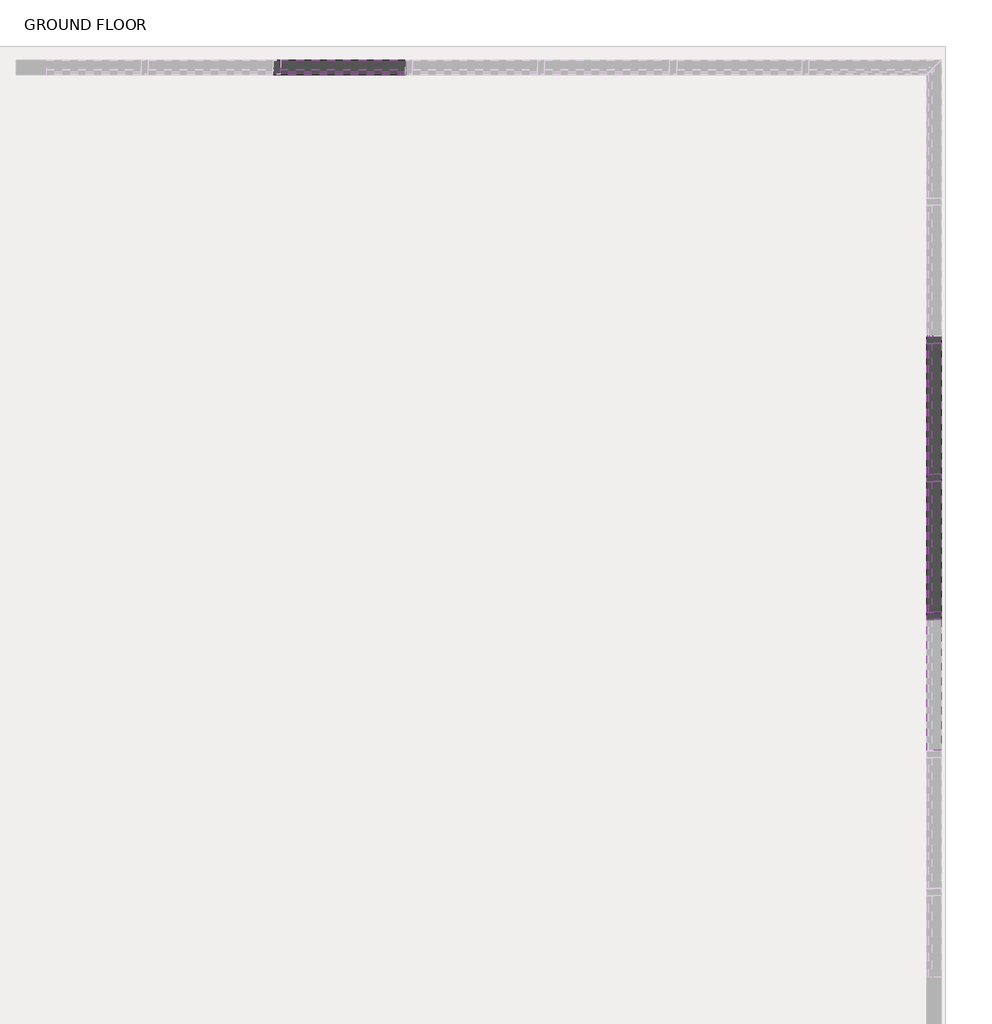
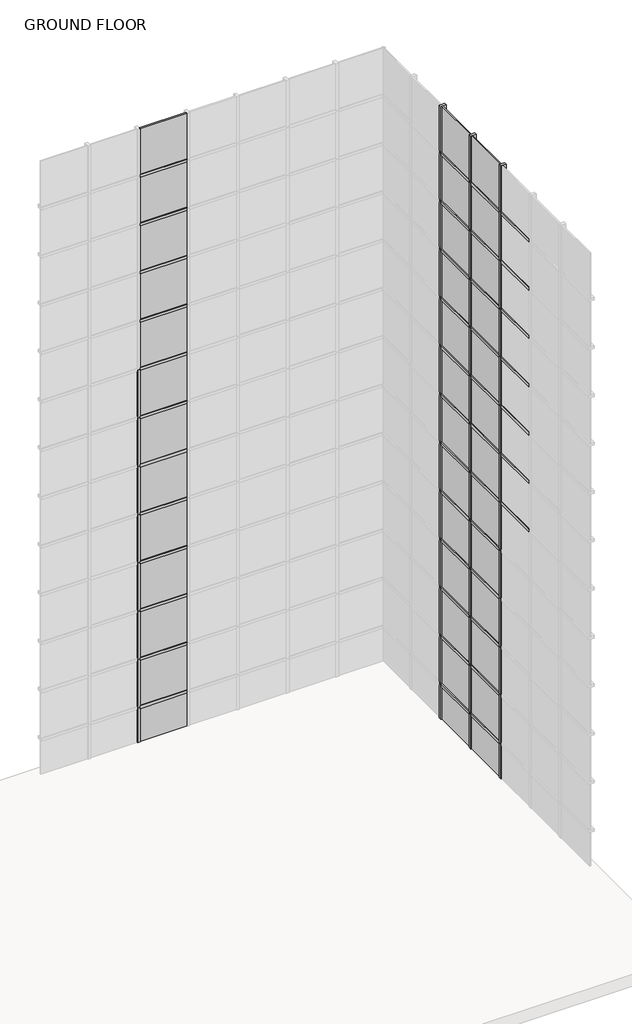
# One storey, part 12 of 16: 90 members, 39 plates.
"""IFC4 building model written with IfcOpenShell, lengths in millimetres."""

from ifc_helpers import new_model, si_unit, origin, place, context, project, spatial, transform, mapped, element, save
from components import member_d518c94e, member_b860638c, member_31fee25f, member_49b1bc66, system_panel_glazed_5cba32e5, system_panel_glazed_49652e9e

model = new_model("IFC4")

# Units and contexts
model_context = context("Model", 3, world=origin())
ifc_project = project(units=[si_unit("LENGTHUNIT", "METRE", prefix="MILLI")], contexts=[model_context])

# Site, building, storey
site = spatial("IfcSite", under=ifc_project)
building = spatial("IfcBuilding", under=site)
storey = spatial("IfcBuildingStorey", under=building, Name="GROUND FLOOR", Elevation=0.0)

# Members
placement = place(None, origin())
member_shape = member_d518c94e(model_context)
element("IfcMember", 1, ObjectType="Rectangular Mullion : 2.5\" x 5\" rectangular", at=placement, inside=storey, context=model_context, shape_type="MappedRepresentation", body=[
    mapped(member_shape, transform((198.8520927, 6370.2261968, 1168.8884615), x_axis=(0.0, 0.0, 1.0), y_axis=(0.0, 1.0, 0.0), z_axis=(-1.0, 0.0, 0.0))),
])
element("IfcMember", 2, ObjectType="Rectangular Mullion : 2.5\" x 5\" rectangular", at=placement, inside=storey, context=model_context, shape_type="MappedRepresentation", body=[
    mapped(member_shape, transform((198.8520927, 6370.2261968, 2369.5269231), x_axis=(0.0, 0.0, 1.0), y_axis=(0.0, 1.0, 0.0), z_axis=(-1.0, 0.0, 0.0))),
])
element("IfcMember", 3, ObjectType="Rectangular Mullion : 2.5\" x 5\" rectangular", at=placement, inside=storey, context=model_context, shape_type="MappedRepresentation", body=[
    mapped(member_shape, transform((198.8520927, 6370.2261968, 3570.1653846), x_axis=(0.0, 0.0, 1.0), y_axis=(0.0, 1.0, 0.0), z_axis=(-1.0, 0.0, 0.0))),
])
element("IfcMember", 4, ObjectType="Rectangular Mullion : 2.5\" x 5\" rectangular", at=placement, inside=storey, context=model_context, shape_type="MappedRepresentation", body=[
    mapped(member_shape, transform((198.8520927, 6370.2261968, 4770.8038462), x_axis=(0.0, 0.0, 1.0), y_axis=(0.0, 1.0, 0.0), z_axis=(-1.0, 0.0, 0.0))),
])
element("IfcMember", 5, ObjectType="Rectangular Mullion : 2.5\" x 5\" rectangular", at=placement, inside=storey, context=model_context, shape_type="MappedRepresentation", body=[
    mapped(member_shape, transform((198.8520927, 6370.2261968, 5971.4423077), x_axis=(0.0, 0.0, 1.0), y_axis=(0.0, 1.0, 0.0), z_axis=(-1.0, 0.0, 0.0))),
])
element("IfcMember", 6, ObjectType="Rectangular Mullion : 2.5\" x 5\" rectangular", at=placement, inside=storey, context=model_context, shape_type="MappedRepresentation", body=[
    mapped(member_shape, transform((198.8520927, 6370.2261968, 7172.0807692), x_axis=(0.0, 0.0, 1.0), y_axis=(0.0, 1.0, 0.0), z_axis=(-1.0, 0.0, 0.0))),
])
element("IfcMember", 7, ObjectType="Rectangular Mullion : 2.5\" x 5\" rectangular", at=placement, inside=storey, context=model_context, shape_type="MappedRepresentation", body=[
    mapped(member_shape, transform((198.8520927, 6370.2261968, 8372.7192308), x_axis=(0.0, 0.0, 1.0), y_axis=(0.0, 1.0, 0.0), z_axis=(-1.0, 0.0, 0.0))),
])
element("IfcMember", 8, ObjectType="Rectangular Mullion : 2.5\" x 5\" rectangular", at=placement, inside=storey, context=model_context, shape_type="MappedRepresentation", body=[
    mapped(member_shape, transform((198.8520927, 6370.2261968, 9573.3576923), x_axis=(0.0, 0.0, 1.0), y_axis=(0.0, 1.0, 0.0), z_axis=(-1.0, 0.0, 0.0))),
])
element("IfcMember", 9, ObjectType="Rectangular Mullion : 2.5\" x 5\" rectangular", at=placement, inside=storey, context=model_context, shape_type="MappedRepresentation", body=[
    mapped(member_shape, transform((198.8520927, 6370.2261968, 10773.9961538), x_axis=(0.0, 0.0, 1.0), y_axis=(0.0, 1.0, 0.0), z_axis=(-1.0, 0.0, 0.0))),
])
element("IfcMember", 10, ObjectType="Rectangular Mullion : 2.5\" x 5\" rectangular", at=placement, inside=storey, context=model_context, shape_type="MappedRepresentation", body=[
    mapped(member_shape, transform((198.8520927, 6370.2261968, 11974.6346154), x_axis=(0.0, 0.0, 1.0), y_axis=(0.0, 1.0, 0.0), z_axis=(-1.0, 0.0, 0.0))),
])
element("IfcMember", 11, ObjectType="Rectangular Mullion : 2.5\" x 5\" rectangular", at=placement, inside=storey, context=model_context, shape_type="MappedRepresentation", body=[
    mapped(member_shape, transform((198.8520927, 6370.2261968, 13175.2730769), x_axis=(0.0, 0.0, 1.0), y_axis=(0.0, 1.0, 0.0), z_axis=(-1.0, 0.0, 0.0))),
])
element("IfcMember", 12, ObjectType="Rectangular Mullion : 2.5\" x 5\" rectangular", at=placement, inside=storey, context=model_context, shape_type="MappedRepresentation", body=[
    mapped(member_shape, transform((198.8520927, 6370.2261968, 14375.9115385), x_axis=(0.0, 0.0, 1.0), y_axis=(0.0, 1.0, 0.0), z_axis=(-1.0, 0.0, 0.0))),
])
member_2_shape = member_b860638c(model_context)
element("IfcMember", 13, ObjectType="Rectangular Mullion : 2.5\" x 5\" rectangular", at=placement, inside=storey, context=model_context, shape_type="MappedRepresentation", body=[
    mapped(member_2_shape, transform((5962.6982466, 1532.7961967, 0.0), x_axis=(0.0, 1.0, 0.0), y_axis=(1.0, 0.0, 0.0), z_axis=(0.0, 0.0, -1.0))),
])
element("IfcMember", 14, ObjectType="Rectangular Mullion : 2.5\" x 5\" rectangular", at=placement, inside=storey, context=model_context, shape_type="MappedRepresentation", body=[
    mapped(member_2_shape, transform((5962.6982466, 2750.0911967, 0.0), x_axis=(0.0, 1.0, 0.0), y_axis=(1.0, 0.0, 0.0), z_axis=(0.0, 0.0, -1.0))),
])
element("IfcMember", 15, ObjectType="Rectangular Mullion : 2.5\" x 5\" rectangular", at=placement, inside=storey, context=model_context, shape_type="MappedRepresentation", body=[
    mapped(member_2_shape, transform((5962.6982466, 3967.3861966, 0.0), x_axis=(0.0, 1.0, 0.0), y_axis=(1.0, 0.0, 0.0), z_axis=(0.0, 0.0, -1.0))),
])
element("IfcMember", 16, ObjectType="Rectangular Mullion : 2.5\" x 5\" rectangular", at=placement, inside=storey, context=model_context, shape_type="MappedRepresentation", body=[
    mapped(member_2_shape, transform((167.1020927, 6370.2261968, 0.0), x_axis=(-1.0, 0.0, 0.0), y_axis=(0.0, 1.0, 0.0), z_axis=(0.0, 0.0, -1.0))),
])
member_3_shape = member_31fee25f(model_context)
element("IfcMember", 17, ObjectType="Rectangular Mullion : 2.5\" x 5\" rectangular", at=placement, inside=storey, context=model_context, shape_type="MappedRepresentation", body=[
    mapped(member_3_shape, transform((5962.6982466, 1532.7961967, 1168.8884615), x_axis=(0.0, 1.0, 0.0), y_axis=(1.0, 0.0, 0.0), z_axis=(0.0, 0.0, -1.0))),
])
element("IfcMember", 18, ObjectType="Rectangular Mullion : 2.5\" x 5\" rectangular", at=placement, inside=storey, context=model_context, shape_type="MappedRepresentation", body=[
    mapped(member_3_shape, transform((5962.6982466, 2750.0911967, 1168.8884615), x_axis=(0.0, 1.0, 0.0), y_axis=(1.0, 0.0, 0.0), z_axis=(0.0, 0.0, -1.0))),
])
element("IfcMember", 19, ObjectType="Rectangular Mullion : 2.5\" x 5\" rectangular", at=placement, inside=storey, context=model_context, shape_type="MappedRepresentation", body=[
    mapped(member_3_shape, transform((5962.6982466, 3967.3861966, 1168.8884615), x_axis=(0.0, 1.0, 0.0), y_axis=(1.0, 0.0, 0.0), z_axis=(0.0, 0.0, -1.0))),
])
element("IfcMember", 20, ObjectType="Rectangular Mullion : 2.5\" x 5\" rectangular", at=placement, inside=storey, context=model_context, shape_type="MappedRepresentation", body=[
    mapped(member_3_shape, transform((5962.6982466, 1532.7961967, 2369.5269231), x_axis=(0.0, 1.0, 0.0), y_axis=(1.0, 0.0, 0.0), z_axis=(0.0, 0.0, -1.0))),
])
element("IfcMember", 21, ObjectType="Rectangular Mullion : 2.5\" x 5\" rectangular", at=placement, inside=storey, context=model_context, shape_type="MappedRepresentation", body=[
    mapped(member_3_shape, transform((5962.6982466, 2750.0911967, 2369.5269231), x_axis=(0.0, 1.0, 0.0), y_axis=(1.0, 0.0, 0.0), z_axis=(0.0, 0.0, -1.0))),
])
element("IfcMember", 22, ObjectType="Rectangular Mullion : 2.5\" x 5\" rectangular", at=placement, inside=storey, context=model_context, shape_type="MappedRepresentation", body=[
    mapped(member_3_shape, transform((5962.6982466, 3967.3861966, 2369.5269231), x_axis=(0.0, 1.0, 0.0), y_axis=(1.0, 0.0, 0.0), z_axis=(0.0, 0.0, -1.0))),
])
element("IfcMember", 23, ObjectType="Rectangular Mullion : 2.5\" x 5\" rectangular", at=placement, inside=storey, context=model_context, shape_type="MappedRepresentation", body=[
    mapped(member_3_shape, transform((5962.6982466, 1532.7961967, 3570.1653846), x_axis=(0.0, 1.0, 0.0), y_axis=(1.0, 0.0, 0.0), z_axis=(0.0, 0.0, -1.0))),
])
element("IfcMember", 24, ObjectType="Rectangular Mullion : 2.5\" x 5\" rectangular", at=placement, inside=storey, context=model_context, shape_type="MappedRepresentation", body=[
    mapped(member_3_shape, transform((5962.6982466, 2750.0911967, 3570.1653846), x_axis=(0.0, 1.0, 0.0), y_axis=(1.0, 0.0, 0.0), z_axis=(0.0, 0.0, -1.0))),
])
element("IfcMember", 25, ObjectType="Rectangular Mullion : 2.5\" x 5\" rectangular", at=placement, inside=storey, context=model_context, shape_type="MappedRepresentation", body=[
    mapped(member_3_shape, transform((5962.6982466, 3967.3861966, 3570.1653846), x_axis=(0.0, 1.0, 0.0), y_axis=(1.0, 0.0, 0.0), z_axis=(0.0, 0.0, -1.0))),
])
element("IfcMember", 26, ObjectType="Rectangular Mullion : 2.5\" x 5\" rectangular", at=placement, inside=storey, context=model_context, shape_type="MappedRepresentation", body=[
    mapped(member_3_shape, transform((5962.6982466, 1532.7961967, 4770.8038462), x_axis=(0.0, 1.0, 0.0), y_axis=(1.0, 0.0, 0.0), z_axis=(0.0, 0.0, -1.0))),
])
element("IfcMember", 27, ObjectType="Rectangular Mullion : 2.5\" x 5\" rectangular", at=placement, inside=storey, context=model_context, shape_type="MappedRepresentation", body=[
    mapped(member_3_shape, transform((5962.6982466, 2750.0911967, 4770.8038462), x_axis=(0.0, 1.0, 0.0), y_axis=(1.0, 0.0, 0.0), z_axis=(0.0, 0.0, -1.0))),
])
element("IfcMember", 28, ObjectType="Rectangular Mullion : 2.5\" x 5\" rectangular", at=placement, inside=storey, context=model_context, shape_type="MappedRepresentation", body=[
    mapped(member_3_shape, transform((5962.6982466, 3967.3861966, 4770.8038462), x_axis=(0.0, 1.0, 0.0), y_axis=(1.0, 0.0, 0.0), z_axis=(0.0, 0.0, -1.0))),
])
element("IfcMember", 29, ObjectType="Rectangular Mullion : 2.5\" x 5\" rectangular", at=placement, inside=storey, context=model_context, shape_type="MappedRepresentation", body=[
    mapped(member_3_shape, transform((5962.6982466, 1532.7961967, 5971.4423077), x_axis=(0.0, 1.0, 0.0), y_axis=(1.0, 0.0, 0.0), z_axis=(0.0, 0.0, -1.0))),
])
element("IfcMember", 30, ObjectType="Rectangular Mullion : 2.5\" x 5\" rectangular", at=placement, inside=storey, context=model_context, shape_type="MappedRepresentation", body=[
    mapped(member_3_shape, transform((5962.6982466, 2750.0911967, 5971.4423077), x_axis=(0.0, 1.0, 0.0), y_axis=(1.0, 0.0, 0.0), z_axis=(0.0, 0.0, -1.0))),
])
element("IfcMember", 31, ObjectType="Rectangular Mullion : 2.5\" x 5\" rectangular", at=placement, inside=storey, context=model_context, shape_type="MappedRepresentation", body=[
    mapped(member_3_shape, transform((5962.6982466, 3967.3861966, 5971.4423077), x_axis=(0.0, 1.0, 0.0), y_axis=(1.0, 0.0, 0.0), z_axis=(0.0, 0.0, -1.0))),
])
element("IfcMember", 32, ObjectType="Rectangular Mullion : 2.5\" x 5\" rectangular", at=placement, inside=storey, context=model_context, shape_type="MappedRepresentation", body=[
    mapped(member_3_shape, transform((5962.6982466, 1532.7961967, 7172.0807692), x_axis=(0.0, 1.0, 0.0), y_axis=(1.0, 0.0, 0.0), z_axis=(0.0, 0.0, -1.0))),
])
element("IfcMember", 33, ObjectType="Rectangular Mullion : 2.5\" x 5\" rectangular", at=placement, inside=storey, context=model_context, shape_type="MappedRepresentation", body=[
    mapped(member_3_shape, transform((5962.6982466, 2750.0911967, 7172.0807692), x_axis=(0.0, 1.0, 0.0), y_axis=(1.0, 0.0, 0.0), z_axis=(0.0, 0.0, -1.0))),
])
element("IfcMember", 34, ObjectType="Rectangular Mullion : 2.5\" x 5\" rectangular", at=placement, inside=storey, context=model_context, shape_type="MappedRepresentation", body=[
    mapped(member_3_shape, transform((5962.6982466, 3967.3861966, 7172.0807692), x_axis=(0.0, 1.0, 0.0), y_axis=(1.0, 0.0, 0.0), z_axis=(0.0, 0.0, -1.0))),
])
element("IfcMember", 35, ObjectType="Rectangular Mullion : 2.5\" x 5\" rectangular", at=placement, inside=storey, context=model_context, shape_type="MappedRepresentation", body=[
    mapped(member_3_shape, transform((5962.6982466, 1532.7961967, 8372.7192308), x_axis=(0.0, 1.0, 0.0), y_axis=(1.0, 0.0, 0.0), z_axis=(0.0, 0.0, -1.0))),
])
element("IfcMember", 36, ObjectType="Rectangular Mullion : 2.5\" x 5\" rectangular", at=placement, inside=storey, context=model_context, shape_type="MappedRepresentation", body=[
    mapped(member_3_shape, transform((5962.6982466, 2750.0911967, 8372.7192308), x_axis=(0.0, 1.0, 0.0), y_axis=(1.0, 0.0, 0.0), z_axis=(0.0, 0.0, -1.0))),
])
element("IfcMember", 37, ObjectType="Rectangular Mullion : 2.5\" x 5\" rectangular", at=placement, inside=storey, context=model_context, shape_type="MappedRepresentation", body=[
    mapped(member_3_shape, transform((5962.6982466, 3967.3861966, 8372.7192308), x_axis=(0.0, 1.0, 0.0), y_axis=(1.0, 0.0, 0.0), z_axis=(0.0, 0.0, -1.0))),
])
element("IfcMember", 38, ObjectType="Rectangular Mullion : 2.5\" x 5\" rectangular", at=placement, inside=storey, context=model_context, shape_type="MappedRepresentation", body=[
    mapped(member_3_shape, transform((5962.6982466, 1532.7961967, 9573.3576923), x_axis=(0.0, 1.0, 0.0), y_axis=(1.0, 0.0, 0.0), z_axis=(0.0, 0.0, -1.0))),
])
element("IfcMember", 39, ObjectType="Rectangular Mullion : 2.5\" x 5\" rectangular", at=placement, inside=storey, context=model_context, shape_type="MappedRepresentation", body=[
    mapped(member_3_shape, transform((5962.6982466, 2750.0911967, 9573.3576923), x_axis=(0.0, 1.0, 0.0), y_axis=(1.0, 0.0, 0.0), z_axis=(0.0, 0.0, -1.0))),
])
element("IfcMember", 40, ObjectType="Rectangular Mullion : 2.5\" x 5\" rectangular", at=placement, inside=storey, context=model_context, shape_type="MappedRepresentation", body=[
    mapped(member_3_shape, transform((5962.6982466, 3967.3861966, 9573.3576923), x_axis=(0.0, 1.0, 0.0), y_axis=(1.0, 0.0, 0.0), z_axis=(0.0, 0.0, -1.0))),
])
element("IfcMember", 41, ObjectType="Rectangular Mullion : 2.5\" x 5\" rectangular", at=placement, inside=storey, context=model_context, shape_type="MappedRepresentation", body=[
    mapped(member_3_shape, transform((5962.6982466, 1532.7961967, 10773.9961538), x_axis=(0.0, 1.0, 0.0), y_axis=(1.0, 0.0, 0.0), z_axis=(0.0, 0.0, -1.0))),
])
element("IfcMember", 42, ObjectType="Rectangular Mullion : 2.5\" x 5\" rectangular", at=placement, inside=storey, context=model_context, shape_type="MappedRepresentation", body=[
    mapped(member_3_shape, transform((5962.6982466, 2750.0911967, 10773.9961538), x_axis=(0.0, 1.0, 0.0), y_axis=(1.0, 0.0, 0.0), z_axis=(0.0, 0.0, -1.0))),
])
element("IfcMember", 43, ObjectType="Rectangular Mullion : 2.5\" x 5\" rectangular", at=placement, inside=storey, context=model_context, shape_type="MappedRepresentation", body=[
    mapped(member_3_shape, transform((5962.6982466, 3967.3861966, 10773.9961538), x_axis=(0.0, 1.0, 0.0), y_axis=(1.0, 0.0, 0.0), z_axis=(0.0, 0.0, -1.0))),
])
element("IfcMember", 44, ObjectType="Rectangular Mullion : 2.5\" x 5\" rectangular", at=placement, inside=storey, context=model_context, shape_type="MappedRepresentation", body=[
    mapped(member_3_shape, transform((5962.6982466, 1532.7961967, 11974.6346154), x_axis=(0.0, 1.0, 0.0), y_axis=(1.0, 0.0, 0.0), z_axis=(0.0, 0.0, -1.0))),
])
element("IfcMember", 45, ObjectType="Rectangular Mullion : 2.5\" x 5\" rectangular", at=placement, inside=storey, context=model_context, shape_type="MappedRepresentation", body=[
    mapped(member_3_shape, transform((5962.6982466, 2750.0911967, 11974.6346154), x_axis=(0.0, 1.0, 0.0), y_axis=(1.0, 0.0, 0.0), z_axis=(0.0, 0.0, -1.0))),
])
element("IfcMember", 46, ObjectType="Rectangular Mullion : 2.5\" x 5\" rectangular", at=placement, inside=storey, context=model_context, shape_type="MappedRepresentation", body=[
    mapped(member_3_shape, transform((5962.6982466, 3967.3861966, 11974.6346154), x_axis=(0.0, 1.0, 0.0), y_axis=(1.0, 0.0, 0.0), z_axis=(0.0, 0.0, -1.0))),
])
element("IfcMember", 47, ObjectType="Rectangular Mullion : 2.5\" x 5\" rectangular", at=placement, inside=storey, context=model_context, shape_type="MappedRepresentation", body=[
    mapped(member_3_shape, transform((5962.6982466, 1532.7961967, 13175.2730769), x_axis=(0.0, 1.0, 0.0), y_axis=(1.0, 0.0, 0.0), z_axis=(0.0, 0.0, -1.0))),
])
element("IfcMember", 48, ObjectType="Rectangular Mullion : 2.5\" x 5\" rectangular", at=placement, inside=storey, context=model_context, shape_type="MappedRepresentation", body=[
    mapped(member_3_shape, transform((5962.6982466, 2750.0911967, 13175.2730769), x_axis=(0.0, 1.0, 0.0), y_axis=(1.0, 0.0, 0.0), z_axis=(0.0, 0.0, -1.0))),
])
element("IfcMember", 49, ObjectType="Rectangular Mullion : 2.5\" x 5\" rectangular", at=placement, inside=storey, context=model_context, shape_type="MappedRepresentation", body=[
    mapped(member_3_shape, transform((5962.6982466, 3967.3861966, 13175.2730769), x_axis=(0.0, 1.0, 0.0), y_axis=(1.0, 0.0, 0.0), z_axis=(0.0, 0.0, -1.0))),
])
element("IfcMember", 50, ObjectType="Rectangular Mullion : 2.5\" x 5\" rectangular", at=placement, inside=storey, context=model_context, shape_type="MappedRepresentation", body=[
    mapped(member_3_shape, transform((167.1020927, 6370.2261968, 1168.8884615), x_axis=(-1.0, 0.0, 0.0), y_axis=(0.0, 1.0, 0.0), z_axis=(0.0, 0.0, -1.0))),
])
element("IfcMember", 51, ObjectType="Rectangular Mullion : 2.5\" x 5\" rectangular", at=placement, inside=storey, context=model_context, shape_type="MappedRepresentation", body=[
    mapped(member_3_shape, transform((167.1020927, 6370.2261968, 2369.5269231), x_axis=(-1.0, 0.0, 0.0), y_axis=(0.0, 1.0, 0.0), z_axis=(0.0, 0.0, -1.0))),
])
element("IfcMember", 52, ObjectType="Rectangular Mullion : 2.5\" x 5\" rectangular", at=placement, inside=storey, context=model_context, shape_type="MappedRepresentation", body=[
    mapped(member_3_shape, transform((167.1020927, 6370.2261968, 3570.1653846), x_axis=(-1.0, 0.0, 0.0), y_axis=(0.0, 1.0, 0.0), z_axis=(0.0, 0.0, -1.0))),
])
element("IfcMember", 53, ObjectType="Rectangular Mullion : 2.5\" x 5\" rectangular", at=placement, inside=storey, context=model_context, shape_type="MappedRepresentation", body=[
    mapped(member_3_shape, transform((167.1020927, 6370.2261968, 4770.8038462), x_axis=(-1.0, 0.0, 0.0), y_axis=(0.0, 1.0, 0.0), z_axis=(0.0, 0.0, -1.0))),
])
element("IfcMember", 54, ObjectType="Rectangular Mullion : 2.5\" x 5\" rectangular", at=placement, inside=storey, context=model_context, shape_type="MappedRepresentation", body=[
    mapped(member_3_shape, transform((167.1020927, 6370.2261968, 5971.4423077), x_axis=(-1.0, 0.0, 0.0), y_axis=(0.0, 1.0, 0.0), z_axis=(0.0, 0.0, -1.0))),
])
element("IfcMember", 55, ObjectType="Rectangular Mullion : 2.5\" x 5\" rectangular", at=placement, inside=storey, context=model_context, shape_type="MappedRepresentation", body=[
    mapped(member_3_shape, transform((167.1020927, 6370.2261968, 7172.0807692), x_axis=(-1.0, 0.0, 0.0), y_axis=(0.0, 1.0, 0.0), z_axis=(0.0, 0.0, -1.0))),
])
element("IfcMember", 56, ObjectType="Rectangular Mullion : 2.5\" x 5\" rectangular", at=placement, inside=storey, context=model_context, shape_type="MappedRepresentation", body=[
    mapped(member_3_shape, transform((167.1020927, 6370.2261968, 8372.7192308), x_axis=(-1.0, 0.0, 0.0), y_axis=(0.0, 1.0, 0.0), z_axis=(0.0, 0.0, -1.0))),
])
element("IfcMember", 57, ObjectType="Rectangular Mullion : 2.5\" x 5\" rectangular", at=placement, inside=storey, context=model_context, shape_type="MappedRepresentation", body=[
    mapped(member_2_shape, transform((5962.6982466, 1532.7961967, 14375.9115385), x_axis=(0.0, 1.0, 0.0), y_axis=(1.0, 0.0, 0.0), z_axis=(0.0, 0.0, -1.0))),
])
element("IfcMember", 58, ObjectType="Rectangular Mullion : 2.5\" x 5\" rectangular", at=placement, inside=storey, context=model_context, shape_type="MappedRepresentation", body=[
    mapped(member_2_shape, transform((5962.6982466, 2750.0911967, 14375.9115385), x_axis=(0.0, 1.0, 0.0), y_axis=(1.0, 0.0, 0.0), z_axis=(0.0, 0.0, -1.0))),
])
element("IfcMember", 59, ObjectType="Rectangular Mullion : 2.5\" x 5\" rectangular", at=placement, inside=storey, context=model_context, shape_type="MappedRepresentation", body=[
    mapped(member_2_shape, transform((5962.6982466, 3967.3861966, 14375.9115385), x_axis=(0.0, 1.0, 0.0), y_axis=(1.0, 0.0, 0.0), z_axis=(0.0, 0.0, -1.0))),
])
member_4_shape = member_49b1bc66(model_context)
element("IfcMember", 60, ObjectType="Rectangular Mullion : 2.5\" x 5\" rectangular", at=placement, inside=storey, context=model_context, shape_type="MappedRepresentation", body=[
    mapped(member_4_shape, transform((5962.6982466, 2718.3411967, 1168.8884615), x_axis=(0.0, 0.0, 1.0), y_axis=(1.0, 0.0, 0.0), z_axis=(0.0, 1.0, 0.0))),
])
element("IfcMember", 61, ObjectType="Rectangular Mullion : 2.5\" x 5\" rectangular", at=placement, inside=storey, context=model_context, shape_type="MappedRepresentation", body=[
    mapped(member_4_shape, transform((5962.6982466, 3935.6361966, 1168.8884615), x_axis=(0.0, 0.0, 1.0), y_axis=(1.0, 0.0, 0.0), z_axis=(0.0, 1.0, 0.0))),
])
element("IfcMember", 62, ObjectType="Rectangular Mullion : 2.5\" x 5\" rectangular", at=placement, inside=storey, context=model_context, shape_type="MappedRepresentation", body=[
    mapped(member_4_shape, transform((5962.6982466, 2718.3411967, 2369.5269231), x_axis=(0.0, 0.0, 1.0), y_axis=(1.0, 0.0, 0.0), z_axis=(0.0, 1.0, 0.0))),
])
element("IfcMember", 63, ObjectType="Rectangular Mullion : 2.5\" x 5\" rectangular", at=placement, inside=storey, context=model_context, shape_type="MappedRepresentation", body=[
    mapped(member_4_shape, transform((5962.6982466, 3935.6361966, 2369.5269231), x_axis=(0.0, 0.0, 1.0), y_axis=(1.0, 0.0, 0.0), z_axis=(0.0, 1.0, 0.0))),
])
element("IfcMember", 64, ObjectType="Rectangular Mullion : 2.5\" x 5\" rectangular", at=placement, inside=storey, context=model_context, shape_type="MappedRepresentation", body=[
    mapped(member_4_shape, transform((5962.6982466, 2718.3411967, 3570.1653846), x_axis=(0.0, 0.0, 1.0), y_axis=(1.0, 0.0, 0.0), z_axis=(0.0, 1.0, 0.0))),
])
element("IfcMember", 65, ObjectType="Rectangular Mullion : 2.5\" x 5\" rectangular", at=placement, inside=storey, context=model_context, shape_type="MappedRepresentation", body=[
    mapped(member_4_shape, transform((5962.6982466, 3935.6361966, 3570.1653846), x_axis=(0.0, 0.0, 1.0), y_axis=(1.0, 0.0, 0.0), z_axis=(0.0, 1.0, 0.0))),
])
element("IfcMember", 66, ObjectType="Rectangular Mullion : 2.5\" x 5\" rectangular", at=placement, inside=storey, context=model_context, shape_type="MappedRepresentation", body=[
    mapped(member_4_shape, transform((5962.6982466, 2718.3411967, 4770.8038462), x_axis=(0.0, 0.0, 1.0), y_axis=(1.0, 0.0, 0.0), z_axis=(0.0, 1.0, 0.0))),
])
element("IfcMember", 67, ObjectType="Rectangular Mullion : 2.5\" x 5\" rectangular", at=placement, inside=storey, context=model_context, shape_type="MappedRepresentation", body=[
    mapped(member_4_shape, transform((5962.6982466, 3935.6361966, 4770.8038462), x_axis=(0.0, 0.0, 1.0), y_axis=(1.0, 0.0, 0.0), z_axis=(0.0, 1.0, 0.0))),
])
element("IfcMember", 68, ObjectType="Rectangular Mullion : 2.5\" x 5\" rectangular", at=placement, inside=storey, context=model_context, shape_type="MappedRepresentation", body=[
    mapped(member_4_shape, transform((5962.6982466, 2718.3411967, 5971.4423077), x_axis=(0.0, 0.0, 1.0), y_axis=(1.0, 0.0, 0.0), z_axis=(0.0, 1.0, 0.0))),
])
element("IfcMember", 69, ObjectType="Rectangular Mullion : 2.5\" x 5\" rectangular", at=placement, inside=storey, context=model_context, shape_type="MappedRepresentation", body=[
    mapped(member_4_shape, transform((5962.6982466, 3935.6361966, 5971.4423077), x_axis=(0.0, 0.0, 1.0), y_axis=(1.0, 0.0, 0.0), z_axis=(0.0, 1.0, 0.0))),
])
element("IfcMember", 70, ObjectType="Rectangular Mullion : 2.5\" x 5\" rectangular", at=placement, inside=storey, context=model_context, shape_type="MappedRepresentation", body=[
    mapped(member_4_shape, transform((5962.6982466, 1501.0461967, 7172.0807692), x_axis=(0.0, 0.0, 1.0), y_axis=(1.0, 0.0, 0.0), z_axis=(0.0, 1.0, 0.0))),
])
element("IfcMember", 71, ObjectType="Rectangular Mullion : 2.5\" x 5\" rectangular", at=placement, inside=storey, context=model_context, shape_type="MappedRepresentation", body=[
    mapped(member_4_shape, transform((5962.6982466, 2718.3411967, 7172.0807692), x_axis=(0.0, 0.0, 1.0), y_axis=(1.0, 0.0, 0.0), z_axis=(0.0, 1.0, 0.0))),
])
element("IfcMember", 72, ObjectType="Rectangular Mullion : 2.5\" x 5\" rectangular", at=placement, inside=storey, context=model_context, shape_type="MappedRepresentation", body=[
    mapped(member_4_shape, transform((5962.6982466, 3935.6361966, 7172.0807692), x_axis=(0.0, 0.0, 1.0), y_axis=(1.0, 0.0, 0.0), z_axis=(0.0, 1.0, 0.0))),
])
element("IfcMember", 73, ObjectType="Rectangular Mullion : 2.5\" x 5\" rectangular", at=placement, inside=storey, context=model_context, shape_type="MappedRepresentation", body=[
    mapped(member_4_shape, transform((5962.6982466, 1501.0461967, 8372.7192308), x_axis=(0.0, 0.0, 1.0), y_axis=(1.0, 0.0, 0.0), z_axis=(0.0, 1.0, 0.0))),
])
element("IfcMember", 74, ObjectType="Rectangular Mullion : 2.5\" x 5\" rectangular", at=placement, inside=storey, context=model_context, shape_type="MappedRepresentation", body=[
    mapped(member_4_shape, transform((5962.6982466, 2718.3411967, 8372.7192308), x_axis=(0.0, 0.0, 1.0), y_axis=(1.0, 0.0, 0.0), z_axis=(0.0, 1.0, 0.0))),
])
element("IfcMember", 75, ObjectType="Rectangular Mullion : 2.5\" x 5\" rectangular", at=placement, inside=storey, context=model_context, shape_type="MappedRepresentation", body=[
    mapped(member_4_shape, transform((5962.6982466, 3935.6361966, 8372.7192308), x_axis=(0.0, 0.0, 1.0), y_axis=(1.0, 0.0, 0.0), z_axis=(0.0, 1.0, 0.0))),
])
element("IfcMember", 76, ObjectType="Rectangular Mullion : 2.5\" x 5\" rectangular", at=placement, inside=storey, context=model_context, shape_type="MappedRepresentation", body=[
    mapped(member_4_shape, transform((5962.6982466, 1501.0461967, 9573.3576923), x_axis=(0.0, 0.0, 1.0), y_axis=(1.0, 0.0, 0.0), z_axis=(0.0, 1.0, 0.0))),
])
element("IfcMember", 77, ObjectType="Rectangular Mullion : 2.5\" x 5\" rectangular", at=placement, inside=storey, context=model_context, shape_type="MappedRepresentation", body=[
    mapped(member_4_shape, transform((5962.6982466, 2718.3411967, 9573.3576923), x_axis=(0.0, 0.0, 1.0), y_axis=(1.0, 0.0, 0.0), z_axis=(0.0, 1.0, 0.0))),
])
element("IfcMember", 78, ObjectType="Rectangular Mullion : 2.5\" x 5\" rectangular", at=placement, inside=storey, context=model_context, shape_type="MappedRepresentation", body=[
    mapped(member_4_shape, transform((5962.6982466, 3935.6361966, 9573.3576923), x_axis=(0.0, 0.0, 1.0), y_axis=(1.0, 0.0, 0.0), z_axis=(0.0, 1.0, 0.0))),
])
element("IfcMember", 79, ObjectType="Rectangular Mullion : 2.5\" x 5\" rectangular", at=placement, inside=storey, context=model_context, shape_type="MappedRepresentation", body=[
    mapped(member_4_shape, transform((5962.6982466, 1501.0461967, 10773.9961538), x_axis=(0.0, 0.0, 1.0), y_axis=(1.0, 0.0, 0.0), z_axis=(0.0, 1.0, 0.0))),
])
element("IfcMember", 80, ObjectType="Rectangular Mullion : 2.5\" x 5\" rectangular", at=placement, inside=storey, context=model_context, shape_type="MappedRepresentation", body=[
    mapped(member_4_shape, transform((5962.6982466, 2718.3411967, 10773.9961538), x_axis=(0.0, 0.0, 1.0), y_axis=(1.0, 0.0, 0.0), z_axis=(0.0, 1.0, 0.0))),
])
element("IfcMember", 81, ObjectType="Rectangular Mullion : 2.5\" x 5\" rectangular", at=placement, inside=storey, context=model_context, shape_type="MappedRepresentation", body=[
    mapped(member_4_shape, transform((5962.6982466, 3935.6361966, 10773.9961538), x_axis=(0.0, 0.0, 1.0), y_axis=(1.0, 0.0, 0.0), z_axis=(0.0, 1.0, 0.0))),
])
element("IfcMember", 82, ObjectType="Rectangular Mullion : 2.5\" x 5\" rectangular", at=placement, inside=storey, context=model_context, shape_type="MappedRepresentation", body=[
    mapped(member_4_shape, transform((5962.6982466, 1501.0461967, 11974.6346154), x_axis=(0.0, 0.0, 1.0), y_axis=(1.0, 0.0, 0.0), z_axis=(0.0, 1.0, 0.0))),
])
element("IfcMember", 83, ObjectType="Rectangular Mullion : 2.5\" x 5\" rectangular", at=placement, inside=storey, context=model_context, shape_type="MappedRepresentation", body=[
    mapped(member_4_shape, transform((5962.6982466, 2718.3411967, 11974.6346154), x_axis=(0.0, 0.0, 1.0), y_axis=(1.0, 0.0, 0.0), z_axis=(0.0, 1.0, 0.0))),
])
element("IfcMember", 84, ObjectType="Rectangular Mullion : 2.5\" x 5\" rectangular", at=placement, inside=storey, context=model_context, shape_type="MappedRepresentation", body=[
    mapped(member_4_shape, transform((5962.6982466, 3935.6361966, 11974.6346154), x_axis=(0.0, 0.0, 1.0), y_axis=(1.0, 0.0, 0.0), z_axis=(0.0, 1.0, 0.0))),
])
element("IfcMember", 85, ObjectType="Rectangular Mullion : 2.5\" x 5\" rectangular", at=placement, inside=storey, context=model_context, shape_type="MappedRepresentation", body=[
    mapped(member_4_shape, transform((5962.6982466, 1501.0461967, 13175.2730769), x_axis=(0.0, 0.0, 1.0), y_axis=(1.0, 0.0, 0.0), z_axis=(0.0, 1.0, 0.0))),
])
element("IfcMember", 86, ObjectType="Rectangular Mullion : 2.5\" x 5\" rectangular", at=placement, inside=storey, context=model_context, shape_type="MappedRepresentation", body=[
    mapped(member_4_shape, transform((5962.6982466, 2718.3411967, 13175.2730769), x_axis=(0.0, 0.0, 1.0), y_axis=(1.0, 0.0, 0.0), z_axis=(0.0, 1.0, 0.0))),
])
element("IfcMember", 87, ObjectType="Rectangular Mullion : 2.5\" x 5\" rectangular", at=placement, inside=storey, context=model_context, shape_type="MappedRepresentation", body=[
    mapped(member_4_shape, transform((5962.6982466, 3935.6361966, 13175.2730769), x_axis=(0.0, 0.0, 1.0), y_axis=(1.0, 0.0, 0.0), z_axis=(0.0, 1.0, 0.0))),
])
element("IfcMember", 88, ObjectType="Rectangular Mullion : 2.5\" x 5\" rectangular", at=placement, inside=storey, context=model_context, shape_type="MappedRepresentation", body=[
    mapped(member_4_shape, transform((5962.6982466, 1501.0461967, 14375.9115385), x_axis=(0.0, 0.0, 1.0), y_axis=(1.0, 0.0, 0.0), z_axis=(0.0, 1.0, 0.0))),
])
element("IfcMember", 89, ObjectType="Rectangular Mullion : 2.5\" x 5\" rectangular", at=placement, inside=storey, context=model_context, shape_type="MappedRepresentation", body=[
    mapped(member_4_shape, transform((5962.6982466, 2718.3411967, 14375.9115385), x_axis=(0.0, 0.0, 1.0), y_axis=(1.0, 0.0, 0.0), z_axis=(0.0, 1.0, 0.0))),
])
element("IfcMember", 90, ObjectType="Rectangular Mullion : 2.5\" x 5\" rectangular", at=placement, inside=storey, context=model_context, shape_type="MappedRepresentation", body=[
    mapped(member_4_shape, transform((5962.6982466, 3935.6361966, 14375.9115385), x_axis=(0.0, 0.0, 1.0), y_axis=(1.0, 0.0, 0.0), z_axis=(0.0, 1.0, 0.0))),
])

# Plates
system_panel_glazed_shape = system_panel_glazed_5cba32e5(model_context)
element("IfcPlate", 91, ObjectType="System Panel : Glazed", at=placement, inside=storey, context=model_context, shape_type="MappedRepresentation", body=[
    mapped(system_panel_glazed_shape, transform((749.836708, 6370.2261968, 0.0), x_axis=(-1.0, 0.0, 0.0), y_axis=(0.0, -1.0, 0.0), z_axis=(0.0, 0.0, 1.0))),
])
element("IfcPlate", 92, ObjectType="System Panel : Glazed", at=placement, inside=storey, context=model_context, shape_type="MappedRepresentation", body=[
    mapped(system_panel_glazed_shape, transform((749.836708, 6370.2261968, 1200.6384615), x_axis=(-1.0, 0.0, 0.0), y_axis=(0.0, -1.0, 0.0), z_axis=(0.0, 0.0, 1.0))),
])
element("IfcPlate", 93, ObjectType="System Panel : Glazed", at=placement, inside=storey, context=model_context, shape_type="MappedRepresentation", body=[
    mapped(system_panel_glazed_shape, transform((749.836708, 6370.2261968, 2401.2769231), x_axis=(-1.0, 0.0, 0.0), y_axis=(0.0, -1.0, 0.0), z_axis=(0.0, 0.0, 1.0))),
])
element("IfcPlate", 94, ObjectType="System Panel : Glazed", at=placement, inside=storey, context=model_context, shape_type="MappedRepresentation", body=[
    mapped(system_panel_glazed_shape, transform((749.836708, 6370.2261968, 3601.9153846), x_axis=(-1.0, 0.0, 0.0), y_axis=(0.0, -1.0, 0.0), z_axis=(0.0, 0.0, 1.0))),
])
element("IfcPlate", 95, ObjectType="System Panel : Glazed", at=placement, inside=storey, context=model_context, shape_type="MappedRepresentation", body=[
    mapped(system_panel_glazed_shape, transform((749.836708, 6370.2261968, 4802.5538462), x_axis=(-1.0, 0.0, 0.0), y_axis=(0.0, -1.0, 0.0), z_axis=(0.0, 0.0, 1.0))),
])
element("IfcPlate", 96, ObjectType="System Panel : Glazed", at=placement, inside=storey, context=model_context, shape_type="MappedRepresentation", body=[
    mapped(system_panel_glazed_shape, transform((749.836708, 6370.2261968, 6003.1923077), x_axis=(-1.0, 0.0, 0.0), y_axis=(0.0, -1.0, 0.0), z_axis=(0.0, 0.0, 1.0))),
])
element("IfcPlate", 97, ObjectType="System Panel : Glazed", at=placement, inside=storey, context=model_context, shape_type="MappedRepresentation", body=[
    mapped(system_panel_glazed_shape, transform((749.836708, 6370.2261968, 7203.8307692), x_axis=(-1.0, 0.0, 0.0), y_axis=(0.0, -1.0, 0.0), z_axis=(0.0, 0.0, 1.0))),
])
element("IfcPlate", 98, ObjectType="System Panel : Glazed", at=placement, inside=storey, context=model_context, shape_type="MappedRepresentation", body=[
    mapped(system_panel_glazed_shape, transform((749.836708, 6370.2261968, 8404.4692308), x_axis=(-1.0, 0.0, 0.0), y_axis=(0.0, -1.0, 0.0), z_axis=(0.0, 0.0, 1.0))),
])
element("IfcPlate", 99, ObjectType="System Panel : Glazed", at=placement, inside=storey, context=model_context, shape_type="MappedRepresentation", body=[
    mapped(system_panel_glazed_shape, transform((749.836708, 6370.2261968, 9605.1076923), x_axis=(-1.0, 0.0, 0.0), y_axis=(0.0, -1.0, 0.0), z_axis=(0.0, 0.0, 1.0))),
])
element("IfcPlate", 100, ObjectType="System Panel : Glazed", at=placement, inside=storey, context=model_context, shape_type="MappedRepresentation", body=[
    mapped(system_panel_glazed_shape, transform((749.836708, 6370.2261968, 10805.7461538), x_axis=(-1.0, 0.0, 0.0), y_axis=(0.0, -1.0, 0.0), z_axis=(0.0, 0.0, 1.0))),
])
element("IfcPlate", 101, ObjectType="System Panel : Glazed", at=placement, inside=storey, context=model_context, shape_type="MappedRepresentation", body=[
    mapped(system_panel_glazed_shape, transform((749.836708, 6370.2261968, 12006.3846154), x_axis=(-1.0, 0.0, 0.0), y_axis=(0.0, -1.0, 0.0), z_axis=(0.0, 0.0, 1.0))),
])
element("IfcPlate", 102, ObjectType="System Panel : Glazed", at=placement, inside=storey, context=model_context, shape_type="MappedRepresentation", body=[
    mapped(system_panel_glazed_shape, transform((749.836708, 6370.2261968, 13207.0230769), x_axis=(-1.0, 0.0, 0.0), y_axis=(0.0, -1.0, 0.0), z_axis=(0.0, 0.0, 1.0))),
])
element("IfcPlate", 103, ObjectType="System Panel : Glazed", at=placement, inside=storey, context=model_context, shape_type="MappedRepresentation", body=[
    mapped(system_panel_glazed_shape, transform((749.836708, 6370.2261968, 14407.6615385), x_axis=(-1.0, 0.0, 0.0), y_axis=(0.0, -1.0, 0.0), z_axis=(0.0, 0.0, 1.0))),
])
system_panel_glazed_2_shape = system_panel_glazed_49652e9e(model_context)
element("IfcPlate", 104, ObjectType="System Panel : Glazed", at=placement, inside=storey, context=model_context, shape_type="MappedRepresentation", body=[
    mapped(system_panel_glazed_2_shape, transform((5962.6982466, 2141.4436967, 0.0), x_axis=(0.0, 1.0, 0.0), y_axis=(-1.0, 0.0, 0.0), z_axis=(0.0, 0.0, 1.0))),
])
element("IfcPlate", 105, ObjectType="System Panel : Glazed", at=placement, inside=storey, context=model_context, shape_type="MappedRepresentation", body=[
    mapped(system_panel_glazed_2_shape, transform((5962.6982466, 3358.7386966, 0.0), x_axis=(0.0, 1.0, 0.0), y_axis=(-1.0, 0.0, 0.0), z_axis=(0.0, 0.0, 1.0))),
])
element("IfcPlate", 106, ObjectType="System Panel : Glazed", at=placement, inside=storey, context=model_context, shape_type="MappedRepresentation", body=[
    mapped(system_panel_glazed_2_shape, transform((5962.6982466, 2141.4436967, 1200.6384615), x_axis=(0.0, 1.0, 0.0), y_axis=(-1.0, 0.0, 0.0), z_axis=(0.0, 0.0, 1.0))),
])
element("IfcPlate", 107, ObjectType="System Panel : Glazed", at=placement, inside=storey, context=model_context, shape_type="MappedRepresentation", body=[
    mapped(system_panel_glazed_2_shape, transform((5962.6982466, 3358.7386966, 1200.6384615), x_axis=(0.0, 1.0, 0.0), y_axis=(-1.0, 0.0, 0.0), z_axis=(0.0, 0.0, 1.0))),
])
element("IfcPlate", 108, ObjectType="System Panel : Glazed", at=placement, inside=storey, context=model_context, shape_type="MappedRepresentation", body=[
    mapped(system_panel_glazed_2_shape, transform((5962.6982466, 2141.4436967, 2401.2769231), x_axis=(0.0, 1.0, 0.0), y_axis=(-1.0, 0.0, 0.0), z_axis=(0.0, 0.0, 1.0))),
])
element("IfcPlate", 109, ObjectType="System Panel : Glazed", at=placement, inside=storey, context=model_context, shape_type="MappedRepresentation", body=[
    mapped(system_panel_glazed_2_shape, transform((5962.6982466, 3358.7386966, 2401.2769231), x_axis=(0.0, 1.0, 0.0), y_axis=(-1.0, 0.0, 0.0), z_axis=(0.0, 0.0, 1.0))),
])
element("IfcPlate", 110, ObjectType="System Panel : Glazed", at=placement, inside=storey, context=model_context, shape_type="MappedRepresentation", body=[
    mapped(system_panel_glazed_2_shape, transform((5962.6982466, 2141.4436967, 3601.9153846), x_axis=(0.0, 1.0, 0.0), y_axis=(-1.0, 0.0, 0.0), z_axis=(0.0, 0.0, 1.0))),
])
element("IfcPlate", 111, ObjectType="System Panel : Glazed", at=placement, inside=storey, context=model_context, shape_type="MappedRepresentation", body=[
    mapped(system_panel_glazed_2_shape, transform((5962.6982466, 3358.7386966, 3601.9153846), x_axis=(0.0, 1.0, 0.0), y_axis=(-1.0, 0.0, 0.0), z_axis=(0.0, 0.0, 1.0))),
])
element("IfcPlate", 112, ObjectType="System Panel : Glazed", at=placement, inside=storey, context=model_context, shape_type="MappedRepresentation", body=[
    mapped(system_panel_glazed_2_shape, transform((5962.6982466, 2141.4436967, 4802.5538462), x_axis=(0.0, 1.0, 0.0), y_axis=(-1.0, 0.0, 0.0), z_axis=(0.0, 0.0, 1.0))),
])
element("IfcPlate", 113, ObjectType="System Panel : Glazed", at=placement, inside=storey, context=model_context, shape_type="MappedRepresentation", body=[
    mapped(system_panel_glazed_2_shape, transform((5962.6982466, 3358.7386966, 4802.5538462), x_axis=(0.0, 1.0, 0.0), y_axis=(-1.0, 0.0, 0.0), z_axis=(0.0, 0.0, 1.0))),
])
element("IfcPlate", 114, ObjectType="System Panel : Glazed", at=placement, inside=storey, context=model_context, shape_type="MappedRepresentation", body=[
    mapped(system_panel_glazed_2_shape, transform((5962.6982466, 2141.4436967, 6003.1923077), x_axis=(0.0, 1.0, 0.0), y_axis=(-1.0, 0.0, 0.0), z_axis=(0.0, 0.0, 1.0))),
])
element("IfcPlate", 115, ObjectType="System Panel : Glazed", at=placement, inside=storey, context=model_context, shape_type="MappedRepresentation", body=[
    mapped(system_panel_glazed_2_shape, transform((5962.6982466, 3358.7386966, 6003.1923077), x_axis=(0.0, 1.0, 0.0), y_axis=(-1.0, 0.0, 0.0), z_axis=(0.0, 0.0, 1.0))),
])
element("IfcPlate", 116, ObjectType="System Panel : Glazed", at=placement, inside=storey, context=model_context, shape_type="MappedRepresentation", body=[
    mapped(system_panel_glazed_2_shape, transform((5962.6982466, 2141.4436967, 7203.8307692), x_axis=(0.0, 1.0, 0.0), y_axis=(-1.0, 0.0, 0.0), z_axis=(0.0, 0.0, 1.0))),
])
element("IfcPlate", 117, ObjectType="System Panel : Glazed", at=placement, inside=storey, context=model_context, shape_type="MappedRepresentation", body=[
    mapped(system_panel_glazed_2_shape, transform((5962.6982466, 3358.7386966, 7203.8307692), x_axis=(0.0, 1.0, 0.0), y_axis=(-1.0, 0.0, 0.0), z_axis=(0.0, 0.0, 1.0))),
])
element("IfcPlate", 118, ObjectType="System Panel : Glazed", at=placement, inside=storey, context=model_context, shape_type="MappedRepresentation", body=[
    mapped(system_panel_glazed_2_shape, transform((5962.6982466, 2141.4436967, 8404.4692308), x_axis=(0.0, 1.0, 0.0), y_axis=(-1.0, 0.0, 0.0), z_axis=(0.0, 0.0, 1.0))),
])
element("IfcPlate", 119, ObjectType="System Panel : Glazed", at=placement, inside=storey, context=model_context, shape_type="MappedRepresentation", body=[
    mapped(system_panel_glazed_2_shape, transform((5962.6982466, 3358.7386966, 8404.4692308), x_axis=(0.0, 1.0, 0.0), y_axis=(-1.0, 0.0, 0.0), z_axis=(0.0, 0.0, 1.0))),
])
element("IfcPlate", 120, ObjectType="System Panel : Glazed", at=placement, inside=storey, context=model_context, shape_type="MappedRepresentation", body=[
    mapped(system_panel_glazed_2_shape, transform((5962.6982466, 2141.4436967, 9605.1076923), x_axis=(0.0, 1.0, 0.0), y_axis=(-1.0, 0.0, 0.0), z_axis=(0.0, 0.0, 1.0))),
])
element("IfcPlate", 121, ObjectType="System Panel : Glazed", at=placement, inside=storey, context=model_context, shape_type="MappedRepresentation", body=[
    mapped(system_panel_glazed_2_shape, transform((5962.6982466, 3358.7386966, 9605.1076923), x_axis=(0.0, 1.0, 0.0), y_axis=(-1.0, 0.0, 0.0), z_axis=(0.0, 0.0, 1.0))),
])
element("IfcPlate", 122, ObjectType="System Panel : Glazed", at=placement, inside=storey, context=model_context, shape_type="MappedRepresentation", body=[
    mapped(system_panel_glazed_2_shape, transform((5962.6982466, 2141.4436967, 10805.7461538), x_axis=(0.0, 1.0, 0.0), y_axis=(-1.0, 0.0, 0.0), z_axis=(0.0, 0.0, 1.0))),
])
element("IfcPlate", 123, ObjectType="System Panel : Glazed", at=placement, inside=storey, context=model_context, shape_type="MappedRepresentation", body=[
    mapped(system_panel_glazed_2_shape, transform((5962.6982466, 3358.7386966, 10805.7461538), x_axis=(0.0, 1.0, 0.0), y_axis=(-1.0, 0.0, 0.0), z_axis=(0.0, 0.0, 1.0))),
])
element("IfcPlate", 124, ObjectType="System Panel : Glazed", at=placement, inside=storey, context=model_context, shape_type="MappedRepresentation", body=[
    mapped(system_panel_glazed_2_shape, transform((5962.6982466, 2141.4436967, 12006.3846154), x_axis=(0.0, 1.0, 0.0), y_axis=(-1.0, 0.0, 0.0), z_axis=(0.0, 0.0, 1.0))),
])
element("IfcPlate", 125, ObjectType="System Panel : Glazed", at=placement, inside=storey, context=model_context, shape_type="MappedRepresentation", body=[
    mapped(system_panel_glazed_2_shape, transform((5962.6982466, 3358.7386966, 12006.3846154), x_axis=(0.0, 1.0, 0.0), y_axis=(-1.0, 0.0, 0.0), z_axis=(0.0, 0.0, 1.0))),
])
element("IfcPlate", 126, ObjectType="System Panel : Glazed", at=placement, inside=storey, context=model_context, shape_type="MappedRepresentation", body=[
    mapped(system_panel_glazed_2_shape, transform((5962.6982466, 2141.4436967, 13207.0230769), x_axis=(0.0, 1.0, 0.0), y_axis=(-1.0, 0.0, 0.0), z_axis=(0.0, 0.0, 1.0))),
])
element("IfcPlate", 127, ObjectType="System Panel : Glazed", at=placement, inside=storey, context=model_context, shape_type="MappedRepresentation", body=[
    mapped(system_panel_glazed_2_shape, transform((5962.6982466, 3358.7386966, 13207.0230769), x_axis=(0.0, 1.0, 0.0), y_axis=(-1.0, 0.0, 0.0), z_axis=(0.0, 0.0, 1.0))),
])
element("IfcPlate", 128, ObjectType="System Panel : Glazed", at=placement, inside=storey, context=model_context, shape_type="MappedRepresentation", body=[
    mapped(system_panel_glazed_2_shape, transform((5962.6982466, 2141.4436967, 14407.6615385), x_axis=(0.0, 1.0, 0.0), y_axis=(-1.0, 0.0, 0.0), z_axis=(0.0, 0.0, 1.0))),
])
element("IfcPlate", 129, ObjectType="System Panel : Glazed", at=placement, inside=storey, context=model_context, shape_type="MappedRepresentation", body=[
    mapped(system_panel_glazed_2_shape, transform((5962.6982466, 3358.7386966, 14407.6615385), x_axis=(0.0, 1.0, 0.0), y_axis=(-1.0, 0.0, 0.0), z_axis=(0.0, 0.0, 1.0))),
])

save(model, "model.ifc")

# Revit data of these elements
# Type "Rectangular Mullion : 2.5\" x 5\" rectangular"
#   built-in parameter 1007304 = 0.416667 (stored number, unit not read)
#   built-in parameter 1007301 = 0.104167 (stored number, unit not read)
#   built-in parameter 1007300 = 0.104167 (stored number, unit not read)
# Type "System Panel : Glazed"
#   Construction Type Id = "GSP4R"
#   Analytic Construction = "1/8 in Pilkington single glazing"
#   Visual Light Transmittance = 0.9
#   Solar Heat Gain Coefficient = 0.86
#   Heat Transfer Coefficient (U) = 1.18115 BTU/(h·ft²·°F)
#   Define Thermal Properties by = 1
# Elements 1, 2, 3, 4, 5, 6, 7, 8, 9, 10, 11, 12, 13, 14, 15, 16, 17, 18, 19, 20, 21, 22, 23, 24, 25, 26, 27, 28, 29, 30, 31, 32, 33, 34, 35, 36, 37, 38, 39, 40, 41, 42, 43, 44, 45, 46, 47, 48, 49, 50, 51, 52, 53, 54, 55, 56, 57, 58, 59, 60, 61, 62, 63, 64, 65, 66, 67, 68, 69, 70, 71, 72, 73, 74, 75, 76, 77, 78, 79, 80, 81, 82, 83, 84, 85, 86, 87, 88, 89, 90 (IfcMember, "Rectangular Mullion : 2.5\" x 5\" rectangular")
#   Phase Created = New Construction
#   Materials on its faces: "Aluminum"
# Elements 91, 92, 93, 94, 95, 96, 97, 98, 99, 100, 101, 102, 103, 104, 105, 106, 107, 108, 109, 110, 111, 112, 113, 114, 115, 116, 117, 118, 119, 120, 121, 122, 123, 124, 125, 126, 127, 128, 129 (IfcPlate, "System Panel : Glazed")
#   Phase Created = New Construction
#   Materials on its faces: "Glass"
# Materials
#   "Aluminum": class "Metal", colour RGB 247 247 247, transparency 0, Description = "Aluminum 6061", Cost = 0
#   "Glass": class "Glass", colour RGB 0 128 192, transparency 0.75, Description = "Soda Lime Glass", Cost = 0
